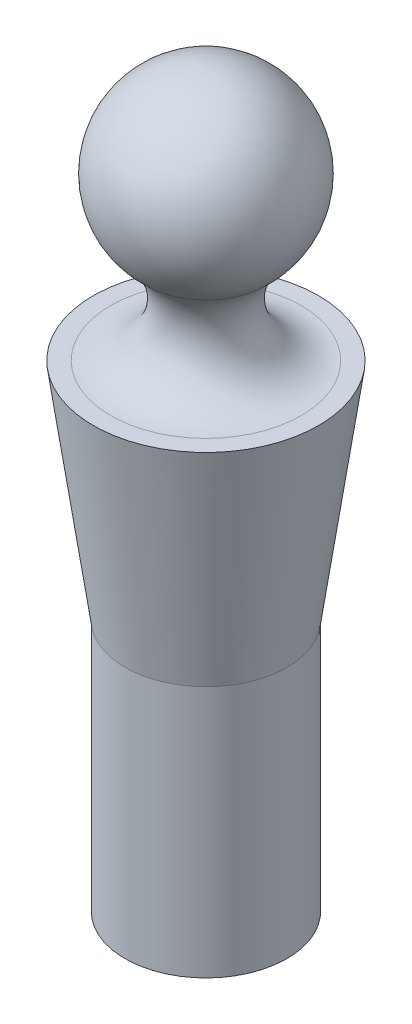
ISO-10303-21;
HEADER;
FILE_DESCRIPTION(('STEP AP214'),'2;1');
FILE_NAME('part.step','',(''),(''),'','','');
FILE_SCHEMA(('AUTOMOTIVE_DESIGN { 1 0 10303 214 1 1 1 1 }'));
ENDSEC;
DATA;
#1=APPLICATION_CONTEXT('core data for automotive mechanical design processes');
#2=APPLICATION_PROTOCOL_DEFINITION('international standard','automotive_design',2000,#1);
#3=PRODUCT_CONTEXT('',#1,'mechanical');
#4=PRODUCT('Part','Part','',(#3));
#5=PRODUCT_RELATED_PRODUCT_CATEGORY('part','',(#4));
#6=PRODUCT_DEFINITION_FORMATION('','',#4);
#7=PRODUCT_DEFINITION_CONTEXT('part definition',#1,'design');
#8=PRODUCT_DEFINITION('design','',#6,#7);
#9=PRODUCT_DEFINITION_SHAPE('','',#8);
#10=(LENGTH_UNIT() NAMED_UNIT(*) SI_UNIT(.MILLI.,.METRE.));
#11=(NAMED_UNIT(*) PLANE_ANGLE_UNIT() SI_UNIT($,.RADIAN.));
#12=(NAMED_UNIT(*) SI_UNIT($,.STERADIAN.) SOLID_ANGLE_UNIT());
#13=UNCERTAINTY_MEASURE_WITH_UNIT(LENGTH_MEASURE(1.E-05),#10,'distance_accuracy_value','');
#14=(GEOMETRIC_REPRESENTATION_CONTEXT(3) GLOBAL_UNCERTAINTY_ASSIGNED_CONTEXT((#13)) GLOBAL_UNIT_ASSIGNED_CONTEXT((#10,
#11,#12)) REPRESENTATION_CONTEXT('',''));
#15=CARTESIAN_POINT('',(0.,0.,0.));
#16=DIRECTION('',(0.,0.,1.));
#17=DIRECTION('',(1.,0.,0.));
#18=AXIS2_PLACEMENT_3D('',#15,#16,#17);
#19=CARTESIAN_POINT('',(9.,-23.3389157487346,0.));
#20=DIRECTION('',(0.,-1.,0.));
#21=DIRECTION('',(0.,0.,-1.));
#22=AXIS2_PLACEMENT_3D('',#19,#20,#21);
#23=PLANE('',#22);
#24=CARTESIAN_POINT('',(0.,-23.3389157487346,0.));
#25=DIRECTION('',(0.,-1.,0.));
#26=DIRECTION('',(0.,0.,-1.));
#27=AXIS2_PLACEMENT_3D('',#24,#25,#26);
#28=CIRCLE('',#27,9.);
#29=CARTESIAN_POINT('',(0.,-23.3389157487346,-9.));
#30=VERTEX_POINT('',#29);
#31=EDGE_CURVE('E10',#30,#30,#28,.T.);
#32=ORIENTED_EDGE('',*,*,#31,.T.);
#33=EDGE_LOOP('',(#32));
#34=FACE_BOUND('',#33,.T.);
#35=ADVANCED_FACE('F40',(#34),#23,.T.);
#36=CARTESIAN_POINT('',(0.,0.,0.));
#37=DIRECTION('',(0.,-1.,0.));
#38=DIRECTION('',(0.,0.,-1.));
#39=AXIS2_PLACEMENT_3D('',#36,#37,#38);
#40=CYLINDRICAL_SURFACE('',#39,9.);
#41=CARTESIAN_POINT('',(0.,4.66108425126535,0.));
#42=DIRECTION('',(0.,-1.,0.));
#43=DIRECTION('',(0.,0.,-1.));
#44=AXIS2_PLACEMENT_3D('',#41,#42,#43);
#45=CIRCLE('',#44,9.);
#46=CARTESIAN_POINT('',(0.,4.66108425126535,-9.));
#47=VERTEX_POINT('',#46);
#48=EDGE_CURVE('E43',#47,#47,#45,.T.);
#49=ORIENTED_EDGE('',*,*,#48,.T.);
#50=EDGE_LOOP('',(#49));
#51=FACE_BOUND('',#50,.T.);
#52=ORIENTED_EDGE('',*,*,#31,.F.);
#53=EDGE_LOOP('',(#52));
#54=FACE_BOUND('',#53,.T.);
#55=ADVANCED_FACE('F75',(#51,#54),#40,.T.);
#56=CARTESIAN_POINT('',(0.,4.66108425126535,0.));
#57=DIRECTION('',(0.,1.,0.));
#58=DIRECTION('',(0.,0.,1.));
#59=AXIS2_PLACEMENT_3D('',#56,#57,#58);
#60=CONICAL_SURFACE('',#59,9.,0.139095941482071);
#61=CARTESIAN_POINT('',(0.,29.6610842512654,0.));
#62=DIRECTION('',(0.,-1.,0.));
#63=DIRECTION('',(0.,0.,-1.));
#64=AXIS2_PLACEMENT_3D('',#61,#62,#63);
#65=CIRCLE('',#64,12.5);
#66=CARTESIAN_POINT('',(0.,29.6610842512654,-12.5));
#67=VERTEX_POINT('',#66);
#68=EDGE_CURVE('E50',#67,#67,#65,.T.);
#69=ORIENTED_EDGE('',*,*,#68,.T.);
#70=EDGE_LOOP('',(#69));
#71=FACE_BOUND('',#70,.T.);
#72=ORIENTED_EDGE('',*,*,#48,.F.);
#73=EDGE_LOOP('',(#72));
#74=FACE_BOUND('',#73,.T.);
#75=ADVANCED_FACE('F78',(#71,#74),#60,.T.);
#76=CARTESIAN_POINT('',(12.5,29.6610842512654,0.));
#77=DIRECTION('',(0.,1.,0.));
#78=DIRECTION('',(0.,0.,1.));
#79=AXIS2_PLACEMENT_3D('',#76,#77,#78);
#80=PLANE('',#79);
#81=CARTESIAN_POINT('',(0.,29.6610842512654,0.));
#82=DIRECTION('',(0.,-1.,0.));
#83=DIRECTION('',(0.,0.,-1.));
#84=AXIS2_PLACEMENT_3D('',#81,#82,#83);
#85=CIRCLE('',#84,10.5830052442584);
#86=CARTESIAN_POINT('',(0.,29.6610842512654,-10.5830052442584));
#87=VERTEX_POINT('',#86);
#88=EDGE_CURVE('E51',#87,#87,#85,.T.);
#89=ORIENTED_EDGE('',*,*,#88,.T.);
#90=EDGE_LOOP('',(#89));
#91=FACE_BOUND('',#90,.T.);
#92=ORIENTED_EDGE('',*,*,#68,.F.);
#93=EDGE_LOOP('',(#92));
#94=FACE_BOUND('',#93,.T.);
#95=ADVANCED_FACE('F66',(#91,#94),#80,.T.);
#96=CARTESIAN_POINT('',(0.,35.6610842512654,0.));
#97=DIRECTION('',(0.,-1.,0.));
#98=DIRECTION('',(0.,0.,-1.));
#99=AXIS2_PLACEMENT_3D('',#96,#97,#98);
#100=TOROIDAL_SURFACE('',#99,10.5830052442584,6.);
#101=CARTESIAN_POINT('',(0.,40.1610842512654,0.));
#102=DIRECTION('',(0.,-1.,0.));
#103=DIRECTION('',(0.,0.,-1.));
#104=AXIS2_PLACEMENT_3D('',#101,#102,#103);
#105=CIRCLE('',#104,6.61437827766149);
#106=CARTESIAN_POINT('',(0.,40.1610842512654,-6.61437827766149));
#107=VERTEX_POINT('',#106);
#108=EDGE_CURVE('E57',#107,#107,#105,.T.);
#109=ORIENTED_EDGE('',*,*,#108,.T.);
#110=EDGE_LOOP('',(#109));
#111=FACE_BOUND('',#110,.T.);
#112=ORIENTED_EDGE('',*,*,#88,.F.);
#113=EDGE_LOOP('',(#112));
#114=FACE_BOUND('',#113,.T.);
#115=ADVANCED_FACE('F58',(#111,#114),#100,.F.);
#116=CARTESIAN_POINT('',(0.,47.6610842512654,0.));
#117=DIRECTION('',(0.,-1.,0.));
#118=DIRECTION('',(1.,0.,0.));
#119=AXIS2_PLACEMENT_3D('',#116,#117,#118);
#120=SPHERICAL_SURFACE('',#119,10.);
#121=ORIENTED_EDGE('',*,*,#108,.F.);
#122=EDGE_LOOP('',(#121));
#123=FACE_BOUND('',#122,.T.);
#124=ADVANCED_FACE('F61',(#123),#120,.T.);
#125=CLOSED_SHELL('',(#35,#55,#75,#95,#115,#124));
#126=MANIFOLD_SOLID_BREP('B2',#125);
#127=ADVANCED_BREP_SHAPE_REPRESENTATION('',(#18,#126),#14);
#128=SHAPE_DEFINITION_REPRESENTATION(#9,#127);
ENDSEC;
END-ISO-10303-21;
